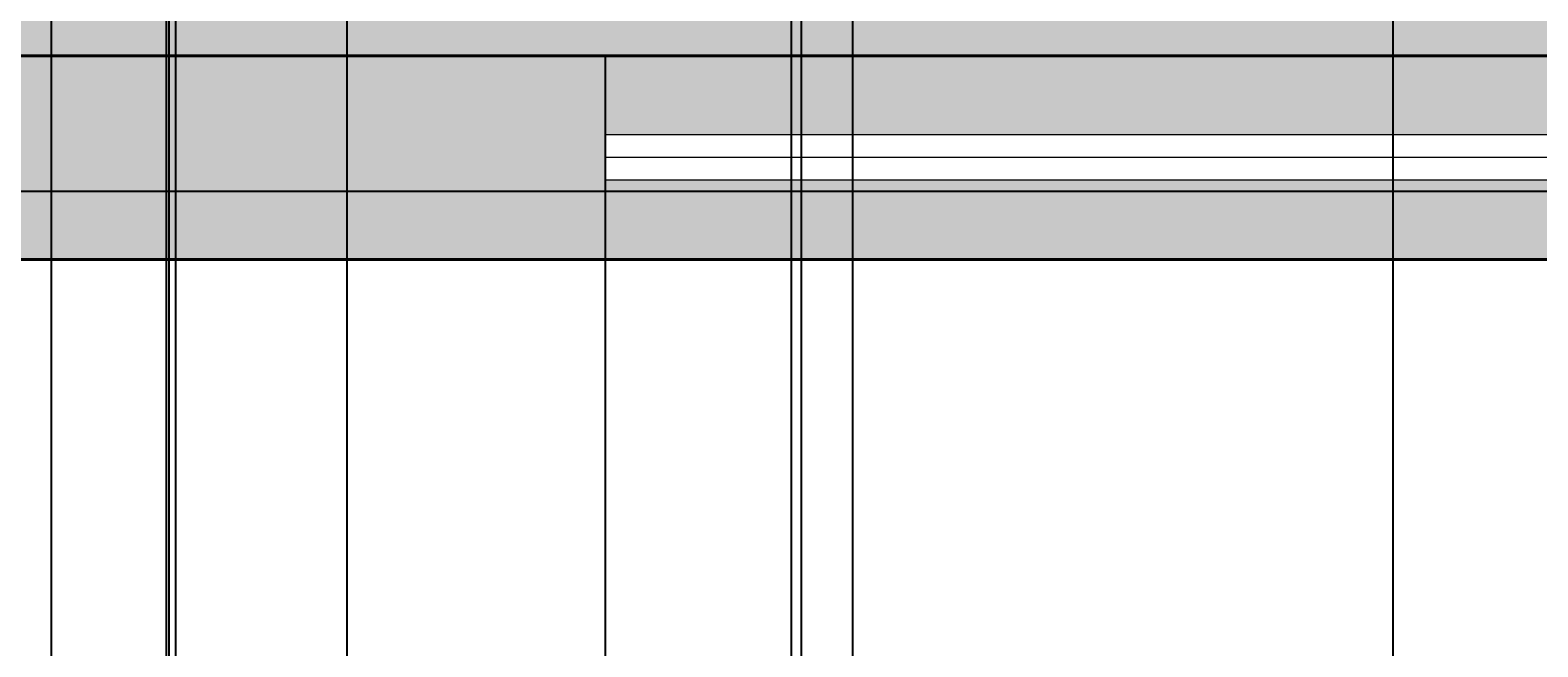
# Model space of a CAD drawing. Units: inches. Extents: x 818 to 1898, y 976 to 2364.
# Tile 74 of 96: x 1305 to 1372, y 2027 to 2054. Entities that reach past the tile are written whole.
import ezdxf

# ---------------------------------------------------------------- set-up
doc = ezdxf.new("R2010")
doc.units = ezdxf.units.IN
doc.header["$LTSCALE"] = 5
doc.header["$MEASUREMENT"] = 0
doc.linetypes.add('HIDDEN', pattern=[0.375, 0.25, -0.125])
for name, color, linetype, lineweight in [('A-ANNO-DIMS', 2, 'Continuous', 18), ('A-FLOR-OVHD', 8, 'HIDDEN', 13), ('A-GLAZ', 4, 'Continuous', 18), ('A-WALL', 7, 'Continuous', 40)]:
    doc.layers.add(name, color=color, linetype=linetype, lineweight=lineweight)
for name, color, linetype, lineweight, true_color in [('A-GLAZ-PATT', 141, 'Continuous', 9, 0xadddf7), ('A-WALL-PATT', 251, 'Continuous', 13, 0x636466), ('L-PLNT-PATT', 114, 'Continuous', 9, 0x139b48)]:
    doc.layers.add(name, color=color, linetype=linetype, lineweight=lineweight, true_color=true_color)
doc.styles.get("Standard").update_dxf_attribs({"font": 'arial.ttf'})
doc.dimstyles.get("Standard").update_dxf_attribs({"dimtxt": 0.18, "dimasz": 0.18, "dimexe": 0.18, "dimexo": 0.0625, "dimgap": 0.09, "dimtad": 0, "dimtih": 1, "dimtoh": 1, "dimdec": 4, "dimzin": 0, "dimdsep": 46, "dimtxsty": 'Standard', "dimcen": 0.09, "dimadec": 0, "dimazin": 0, "dimtfac": 1, "dimtdec": 4, "dimtofl": 0, "dimtmove": 0, "dimatfit": 3, "dimfxl": 1, "dimtolj": 1, "dimtzin": 0, "dimarcsym": 0})

# ---------------------------------------------------------------- blocks, each defined once
blk = doc.blocks.new('*D61')
at = {"layer": 'A-ANNO-DIMS', "color": 0, "lineweight": -2, "ltscale": 5, "transparency": 16777216}
for p, q in [((1071.725, 1203.027), (1071.725, 2363.873)), ((1071.905, 2363.693), (1250.936, 2363.693)), ((1430.545, 2363.693), (1251.514, 2363.693)), ((1430.725, 1203.027), (1430.725, 2363.873))]:
    blk.add_line(p, q, dxfattribs=at)
at = {"layer": 'A-ANNO-DIMS', "color": 0, "ltscale": 5, "transparency": 16777216}
for points in [[(1071.905, 2363.723), (1071.905, 2363.663), (1071.725, 2363.693)], [(1430.545, 2363.723), (1430.545, 2363.663), (1430.725, 2363.693)]]:
    blk.add_solid(points, dxfattribs=at)
at = {"layer": 'Defpoints', "color": 0, "ltscale": 5, "transparency": 16777216}
for p in [(1430.725, 2363.693), (1071.725, 1202.964), (1430.725, 1202.964)]:
    blk.add_point(p, dxfattribs=at)
at = {"layer": 'A-ANNO-DIMS', "color": 0, "ltscale": 5, "transparency": 16777216, "insert": (1251.225, 2363.693), "char_height": 0.18, "attachment_point": 5}
blk.add_mtext('\\A1;359', dxfattribs=at)
blk = doc.blocks.new('*D64')
at = {"layer": 'A-ANNO-DIMS', "color": 0, "lineweight": -2, "ltscale": 5, "transparency": 16777216}
for p, q in [((1197.725, 1501.141), (1197.725, 2363.873)), ((1197.905, 2363.693), (1313.935, 2363.693)), ((1430.545, 2363.693), (1314.516, 2363.693)), ((1430.725, 1501.141), (1430.725, 2363.873))]:
    blk.add_line(p, q, dxfattribs=at)
at = {"layer": 'A-ANNO-DIMS', "color": 0, "ltscale": 5, "transparency": 16777216}
for points in [[(1197.905, 2363.723), (1197.905, 2363.663), (1197.725, 2363.693)], [(1430.545, 2363.723), (1430.545, 2363.663), (1430.725, 2363.693)]]:
    blk.add_solid(points, dxfattribs=at)
at = {"layer": 'Defpoints', "color": 0, "ltscale": 5, "transparency": 16777216}
for p in [(1430.725, 2363.693), (1197.725, 1501.078), (1430.725, 1501.078)]:
    blk.add_point(p, dxfattribs=at)
at = {"layer": 'A-ANNO-DIMS', "color": 0, "ltscale": 5, "transparency": 16777216, "insert": (1314.225, 2363.693), "char_height": 0.18, "attachment_point": 5}
blk.add_mtext('\\A1;233', dxfattribs=at)
blk = doc.blocks.new('*D85')
at = {"layer": 'A-ANNO-DIMS', "color": 0, "lineweight": -2, "ltscale": 5, "transparency": 16777216}
for p, q in [((1258.788, 2053.078), (1897.916, 2053.078)), ((1897.736, 2052.898), (1897.736, 1876.76)), ((1897.736, 1700.258), (1897.736, 1876.396)), ((1258.788, 1700.078), (1897.916, 1700.078))]:
    blk.add_line(p, q, dxfattribs=at)
at = {"layer": 'A-ANNO-DIMS', "color": 0, "ltscale": 5, "transparency": 16777216}
for points in [[(1897.706, 2052.898), (1897.766, 2052.898), (1897.736, 2053.078)], [(1897.706, 1700.258), (1897.766, 1700.258), (1897.736, 1700.078)]]:
    blk.add_solid(points, dxfattribs=at)
at = {"layer": 'Defpoints', "color": 0, "ltscale": 5, "transparency": 16777216}
for p in [(1258.725, 2053.078), (1897.736, 2053.078), (1258.725, 1700.078)]:
    blk.add_point(p, dxfattribs=at)
at = {"layer": 'A-ANNO-DIMS', "color": 0, "ltscale": 5, "transparency": 16777216, "insert": (1897.736, 1876.578), "char_height": 0.18, "attachment_point": 5}
blk.add_mtext('\\A1;353', dxfattribs=at)
blk = doc.blocks.new('*D86')
at = {"layer": 'A-ANNO-DIMS', "color": 0, "lineweight": -2, "ltscale": 5, "transparency": 16777216}
for p, q in [((1258.725, 2053.141), (1258.725, 2363.873)), ((1258.905, 2363.693), (1486.433, 2363.693)), ((1714.545, 2363.693), (1487.018, 2363.693)), ((1714.725, 2053.141), (1714.725, 2363.873))]:
    blk.add_line(p, q, dxfattribs=at)
at = {"layer": 'A-ANNO-DIMS', "color": 0, "ltscale": 5, "transparency": 16777216}
for points in [[(1258.905, 2363.723), (1258.905, 2363.663), (1258.725, 2363.693)], [(1714.545, 2363.723), (1714.545, 2363.663), (1714.725, 2363.693)]]:
    blk.add_solid(points, dxfattribs=at)
at = {"layer": 'Defpoints', "color": 0, "ltscale": 5, "transparency": 16777216}
for p in [(1714.725, 2363.693), (1258.725, 2053.078), (1714.725, 2053.078)]:
    blk.add_point(p, dxfattribs=at)
at = {"layer": 'A-ANNO-DIMS', "color": 0, "ltscale": 5, "transparency": 16777216, "insert": (1486.725, 2363.693), "char_height": 0.18, "attachment_point": 5}
blk.add_mtext('\\A1;456', dxfattribs=at)
blk = doc.blocks.new('*D97')
at = {"layer": 'A-ANNO-DIMS', "color": 0, "lineweight": -2, "ltscale": 5, "transparency": 16777216}
for p, q in [((1284.17, 1071.118), (1284.17, 2363.873)), ((1284.35, 2363.693), (1310.962, 2363.693)), ((1338.361, 2363.693), (1311.749, 2363.693)), ((1338.541, 1071.118), (1338.541, 2363.873))]:
    blk.add_line(p, q, dxfattribs=at)
at = {"layer": 'A-ANNO-DIMS', "color": 0, "ltscale": 5, "transparency": 16777216}
for points in [[(1284.35, 2363.723), (1284.35, 2363.663), (1284.17, 2363.693)], [(1338.361, 2363.723), (1338.361, 2363.663), (1338.541, 2363.693)]]:
    blk.add_solid(points, dxfattribs=at)
at = {"layer": 'Defpoints', "color": 0, "ltscale": 5, "transparency": 16777216}
for p in [(1338.541, 2363.693), (1284.17, 1071.055), (1338.541, 1071.055)]:
    blk.add_point(p, dxfattribs=at)
at = {"layer": 'A-ANNO-DIMS', "color": 0, "ltscale": 5, "transparency": 16777216, "insert": (1311.355, 2363.693), "char_height": 0.18, "attachment_point": 5}
blk.add_mtext('\\A1;54.37', dxfattribs=at)
blk = doc.blocks.new('*D98')
at = {"layer": 'A-ANNO-DIMS', "color": 0, "lineweight": -2, "ltscale": 5, "transparency": 16777216}
for p, q in [((1338.541, 1071.118), (1338.541, 2363.873)), ((1338.721, 2363.693), (1364.815, 2363.693)), ((1391.696, 2363.693), (1365.602, 2363.693)), ((1391.876, 1071.118), (1391.876, 2363.873))]:
    blk.add_line(p, q, dxfattribs=at)
at = {"layer": 'A-ANNO-DIMS', "color": 0, "ltscale": 5, "transparency": 16777216}
for points in [[(1338.721, 2363.723), (1338.721, 2363.663), (1338.541, 2363.693)], [(1391.696, 2363.723), (1391.696, 2363.663), (1391.876, 2363.693)]]:
    blk.add_solid(points, dxfattribs=at)
at = {"layer": 'Defpoints', "color": 0, "ltscale": 5, "transparency": 16777216}
for p in [(1391.876, 2363.693), (1338.541, 1071.055), (1391.876, 1071.055)]:
    blk.add_point(p, dxfattribs=at)
at = {"layer": 'A-ANNO-DIMS', "color": 0, "ltscale": 5, "transparency": 16777216, "insert": (1365.208, 2363.693), "char_height": 0.18, "attachment_point": 5}
blk.add_mtext('\\A1;53.33', dxfattribs=at)
blk = doc.blocks.new('*D165')
at = {"layer": 'A-ANNO-DIMS', "color": 0, "lineweight": -2, "ltscale": 5, "transparency": 16777216}
for p, q in [((1283.818, 1510.141), (1283.818, 2363.873)), ((1283.998, 2363.693), (1324.088, 2363.693)), ((1364.966, 2363.693), (1324.876, 2363.693)), ((1365.146, 1510.141), (1365.146, 2363.873))]:
    blk.add_line(p, q, dxfattribs=at)
at = {"layer": 'A-ANNO-DIMS', "color": 0, "ltscale": 5, "transparency": 16777216}
for points in [[(1283.998, 2363.723), (1283.998, 2363.663), (1283.818, 2363.693)], [(1364.966, 2363.723), (1364.966, 2363.663), (1365.146, 2363.693)]]:
    blk.add_solid(points, dxfattribs=at)
at = {"layer": 'Defpoints', "color": 0, "ltscale": 5, "transparency": 16777216}
for p in [(1365.146, 2363.693), (1283.818, 1510.078), (1365.146, 1510.078)]:
    blk.add_point(p, dxfattribs=at)
at = {"layer": 'A-ANNO-DIMS', "color": 0, "ltscale": 5, "transparency": 16777216, "insert": (1324.482, 2363.693), "char_height": 0.18, "attachment_point": 5}
blk.add_mtext('\\A1;81.33', dxfattribs=at)
blk = doc.blocks.new('*D207')
at = {"layer": 'A-ANNO-DIMS', "color": 0, "lineweight": -2, "ltscale": 5, "transparency": 16777216}
for p, q in [((1590.663, 2044.078), (818.026, 2044.078)), ((818.206, 2043.898), (818.206, 2027.76)), ((818.206, 2011.258), (818.206, 2027.396)), ((1590.663, 2011.078), (818.026, 2011.078))]:
    blk.add_line(p, q, dxfattribs=at)
at = {"layer": 'A-ANNO-DIMS', "color": 0, "ltscale": 5, "transparency": 16777216}
for points in [[(818.176, 2043.898), (818.236, 2043.898), (818.206, 2044.078)], [(818.176, 2011.258), (818.236, 2011.258), (818.206, 2011.078)]]:
    blk.add_solid(points, dxfattribs=at)
at = {"layer": 'Defpoints', "color": 0, "ltscale": 5, "transparency": 16777216}
for p in [(818.206, 2044.078), (1590.725, 2044.078), (1590.725, 2011.078)]:
    blk.add_point(p, dxfattribs=at)
at = {"layer": 'A-ANNO-DIMS', "color": 0, "ltscale": 5, "transparency": 16777216, "insert": (818.206, 2027.578), "char_height": 0.18, "attachment_point": 5}
blk.add_mtext('\\A1;33', dxfattribs=at)
blk = doc.blocks.new('*D235')
at = {"layer": 'A-ANNO-DIMS', "color": 0, "lineweight": -2, "ltscale": 5, "transparency": 16777216}
for p, q in [((1310.908, 2026.27), (1310.908, 2363.873)), ((1311.088, 2363.693), (1324.485, 2363.693)), ((1338.812, 2363.693), (1325.414, 2363.693)), ((1338.992, 2026.27), (1338.992, 2363.873))]:
    blk.add_line(p, q, dxfattribs=at)
at = {"layer": 'A-ANNO-DIMS', "color": 0, "ltscale": 5, "transparency": 16777216}
for points in [[(1311.088, 2363.723), (1311.088, 2363.663), (1310.908, 2363.693)], [(1338.812, 2363.723), (1338.812, 2363.663), (1338.992, 2363.693)]]:
    blk.add_solid(points, dxfattribs=at)
at = {"layer": 'Defpoints', "color": 0, "ltscale": 5, "transparency": 16777216}
for p in [(1338.992, 2363.693), (1310.908, 2026.207), (1338.992, 2026.207)]:
    blk.add_point(p, dxfattribs=at)
at = {"layer": 'A-ANNO-DIMS', "color": 0, "ltscale": 5, "transparency": 16777216, "insert": (1324.95, 2363.693), "char_height": 0.18, "attachment_point": 5}
blk.add_mtext('\\A1;28.084', dxfattribs=at)
blk = doc.blocks.new('*D252')
at = {"layer": 'A-ANNO-DIMS', "color": 0, "lineweight": -2, "ltscale": 5, "transparency": 16777216}
for p, q in [((1330.305, 2053.016), (1330.305, 975.663)), ((1388.031, 2053.016), (1388.031, 975.663)), ((1330.485, 975.843), (1358.775, 975.843)), ((1387.851, 975.843), (1359.562, 975.843))]:
    blk.add_line(p, q, dxfattribs=at)
at = {"layer": 'A-ANNO-DIMS', "color": 0, "ltscale": 5, "transparency": 16777216}
for points in [[(1330.485, 975.873), (1330.485, 975.813), (1330.305, 975.843)], [(1387.851, 975.873), (1387.851, 975.813), (1388.031, 975.843)]]:
    blk.add_solid(points, dxfattribs=at)
at = {"layer": 'Defpoints', "color": 0, "ltscale": 5, "transparency": 16777216}
for p in [(1330.305, 2053.078), (1388.031, 2053.078), (1388.031, 975.843)]:
    blk.add_point(p, dxfattribs=at)
at = {"layer": 'A-ANNO-DIMS', "color": 0, "ltscale": 5, "transparency": 16777216, "insert": (1359.168, 975.843), "char_height": 0.18, "attachment_point": 5}
blk.add_mtext('\\A1;57.73', dxfattribs=at)
blk = doc.blocks.new('*D254')
at = {"layer": 'A-ANNO-DIMS', "color": 0, "lineweight": -2, "ltscale": 5, "transparency": 16777216}
for p, q in [((1267.725, 2044.016), (1267.725, 975.663)), ((1330.305, 2044.016), (1330.305, 975.663)), ((1267.905, 975.843), (1298.621, 975.843)), ((1330.125, 975.843), (1299.409, 975.843))]:
    blk.add_line(p, q, dxfattribs=at)
at = {"layer": 'A-ANNO-DIMS', "color": 0, "ltscale": 5, "transparency": 16777216}
for points in [[(1267.905, 975.873), (1267.905, 975.813), (1267.725, 975.843)], [(1330.125, 975.873), (1330.125, 975.813), (1330.305, 975.843)]]:
    blk.add_solid(points, dxfattribs=at)
at = {"layer": 'Defpoints', "color": 0, "ltscale": 5, "transparency": 16777216}
for p in [(1267.725, 2044.078), (1330.305, 2044.078), (1330.305, 975.843)]:
    blk.add_point(p, dxfattribs=at)
at = {"layer": 'A-ANNO-DIMS', "color": 0, "ltscale": 5, "transparency": 16777216, "insert": (1299.015, 975.843), "char_height": 0.18, "attachment_point": 5}
blk.add_mtext('\\A1;62.58', dxfattribs=at)
blk = doc.blocks.new('*D257')
at = {"layer": 'A-ANNO-DIMS', "color": 0, "lineweight": -2, "ltscale": 5, "transparency": 16777216}
for p, q in [((1399.573, 2077.188), (818.026, 2077.188)), ((818.206, 2077.008), (818.206, 2065.314)), ((818.206, 2053.258), (818.206, 2064.953)), ((1399.573, 2053.078), (818.026, 2053.078))]:
    blk.add_line(p, q, dxfattribs=at)
at = {"layer": 'A-ANNO-DIMS', "color": 0, "ltscale": 5, "transparency": 16777216}
for points in [[(818.176, 2077.008), (818.236, 2077.008), (818.206, 2077.188)], [(818.176, 2053.258), (818.236, 2053.258), (818.206, 2053.078)]]:
    blk.add_solid(points, dxfattribs=at)
at = {"layer": 'Defpoints', "color": 0, "ltscale": 5, "transparency": 16777216}
for p in [(818.206, 2077.188), (1399.636, 2077.188), (1399.636, 2053.078)]:
    blk.add_point(p, dxfattribs=at)
at = {"layer": 'A-ANNO-DIMS', "color": 0, "ltscale": 5, "transparency": 16777216, "insert": (818.206, 2065.133), "char_height": 0.18, "attachment_point": 5}
blk.add_mtext('\\A1;24.11', dxfattribs=at)
blk = doc.blocks.new('*D266')
at = {"layer": 'A-ANNO-DIMS', "color": 0, "lineweight": -2, "ltscale": 5, "transparency": 16777216}
for p, q in [((1780.439, 2053.078), (818.026, 2053.078)), ((818.206, 2052.898), (818.206, 2050.26)), ((818.206, 2047.258), (818.206, 2049.896)), ((1780.439, 2047.078), (818.026, 2047.078))]:
    blk.add_line(p, q, dxfattribs=at)
at = {"layer": 'A-ANNO-DIMS', "color": 0, "ltscale": 5, "transparency": 16777216}
for points in [[(818.176, 2052.898), (818.236, 2052.898), (818.206, 2053.078)], [(818.176, 2047.258), (818.236, 2047.258), (818.206, 2047.078)]]:
    blk.add_solid(points, dxfattribs=at)
at = {"layer": 'Defpoints', "color": 0, "ltscale": 5, "transparency": 16777216}
for p in [(1780.502, 2053.078), (818.206, 2047.078), (1780.502, 2047.078)]:
    blk.add_point(p, dxfattribs=at)
at = {"layer": 'A-ANNO-DIMS', "color": 0, "ltscale": 5, "transparency": 16777216, "insert": (818.206, 2050.078), "char_height": 0.18, "attachment_point": 5}
blk.add_mtext('\\A1;6', dxfattribs=at)
blk = doc.blocks.new('*D269')
at = {"layer": 'A-ANNO-DIMS', "color": 0, "lineweight": -2, "ltscale": 5, "transparency": 16777216}
for p, q in [((1246.938, 1534.141), (1246.938, 2363.873)), ((1247.118, 2363.693), (1293.706, 2363.693)), ((1341.079, 2363.693), (1294.491, 2363.693)), ((1341.259, 1534.141), (1341.259, 2363.873))]:
    blk.add_line(p, q, dxfattribs=at)
at = {"layer": 'A-ANNO-DIMS', "color": 0, "ltscale": 5, "transparency": 16777216}
for points in [[(1247.118, 2363.723), (1247.118, 2363.663), (1246.938, 2363.693)], [(1341.079, 2363.723), (1341.079, 2363.663), (1341.259, 2363.693)]]:
    blk.add_solid(points, dxfattribs=at)
at = {"layer": 'Defpoints', "color": 0, "ltscale": 5, "transparency": 16777216}
for p in [(1341.259, 2363.693), (1246.938, 1534.078), (1341.259, 1534.078)]:
    blk.add_point(p, dxfattribs=at)
at = {"layer": 'A-ANNO-DIMS', "color": 0, "ltscale": 5, "transparency": 16777216, "insert": (1294.099, 2363.693), "char_height": 0.18, "attachment_point": 5}
blk.add_mtext('\\A1;94.32', dxfattribs=at)
blk = doc.blocks.new('*D274')
at = {"layer": 'A-ANNO-DIMS', "color": 0, "lineweight": -2, "ltscale": 5, "transparency": 16777216}
for p, q in [((1311.025, 1897.929), (1311.025, 2363.873)), ((1311.205, 2363.693), (1344.007, 2363.693)), ((1377.599, 2363.693), (1344.797, 2363.693)), ((1377.779, 1897.929), (1377.779, 2363.873))]:
    blk.add_line(p, q, dxfattribs=at)
at = {"layer": 'A-ANNO-DIMS', "color": 0, "ltscale": 5, "transparency": 16777216}
for points in [[(1311.205, 2363.723), (1311.205, 2363.663), (1311.025, 2363.693)], [(1377.599, 2363.723), (1377.599, 2363.663), (1377.779, 2363.693)]]:
    blk.add_solid(points, dxfattribs=at)
at = {"layer": 'Defpoints', "color": 0, "ltscale": 5, "transparency": 16777216}
for p in [(1377.779, 2363.693), (1311.025, 1897.866), (1377.779, 1897.866)]:
    blk.add_point(p, dxfattribs=at)
at = {"layer": 'A-ANNO-DIMS', "color": 0, "ltscale": 5, "transparency": 16777216, "insert": (1344.402, 2363.693), "char_height": 0.18, "attachment_point": 5}
blk.add_mtext('\\A1;66.75', dxfattribs=at)
blk = doc.blocks.new('*D281')
at = {"layer": 'A-ANNO-DIMS', "color": 0, "lineweight": -2, "ltscale": 5, "transparency": 16777216}
for p, q in [((1250.303, 1913.703), (1250.303, 2363.873)), ((1250.483, 2363.693), (1420.121, 2363.693)), ((1590.545, 2363.693), (1420.907, 2363.693)), ((1590.725, 2011.141), (1590.725, 2363.873))]:
    blk.add_line(p, q, dxfattribs=at)
at = {"layer": 'A-ANNO-DIMS', "color": 0, "ltscale": 5, "transparency": 16777216}
for points in [[(1250.483, 2363.723), (1250.483, 2363.663), (1250.303, 2363.693)], [(1590.545, 2363.723), (1590.545, 2363.663), (1590.725, 2363.693)]]:
    blk.add_solid(points, dxfattribs=at)
at = {"layer": 'Defpoints', "color": 0, "ltscale": 5, "transparency": 16777216}
for p in [(1590.725, 2363.693), (1590.725, 2011.078), (1250.303, 1913.64)]:
    blk.add_point(p, dxfattribs=at)
at = {"layer": 'A-ANNO-DIMS', "color": 0, "ltscale": 5, "transparency": 16777216, "insert": (1420.514, 2363.693), "char_height": 0.18, "attachment_point": 5}
blk.add_mtext('\\A1;340.4', dxfattribs=at)
blk = doc.blocks.new('*D286')
at = {"layer": 'A-ANNO-DIMS', "color": 0, "lineweight": -2, "ltscale": 5, "transparency": 16777216}
for p, q in [((1305.828, 1851.971), (1305.828, 2363.873)), ((1306.008, 2363.693), (1308.184, 2363.693)), ((1311.147, 2363.693), (1308.971, 2363.693)), ((1311.327, 1853.812), (1311.327, 2363.873))]:
    blk.add_line(p, q, dxfattribs=at)
at = {"layer": 'A-ANNO-DIMS', "color": 0, "ltscale": 5, "transparency": 16777216}
for points in [[(1306.008, 2363.723), (1306.008, 2363.663), (1305.828, 2363.693)], [(1311.147, 2363.723), (1311.147, 2363.663), (1311.327, 2363.693)]]:
    blk.add_solid(points, dxfattribs=at)
at = {"layer": 'Defpoints', "color": 0, "ltscale": 5, "transparency": 16777216}
for p in [(1305.828, 2363.693), (1311.327, 1853.75), (1305.828, 1851.908)]:
    blk.add_point(p, dxfattribs=at)
at = {"layer": 'A-ANNO-DIMS', "color": 0, "ltscale": 5, "transparency": 16777216, "insert": (1308.577, 2363.693), "char_height": 0.18, "attachment_point": 5}
blk.add_mtext('\\A1;5.499', dxfattribs=at)
blk = doc.blocks.new('*D290')
at = {"layer": 'A-ANNO-DIMS', "color": 0, "lineweight": -2, "ltscale": 5, "transparency": 16777216}
for p, q in [((1302.983, 1599.435), (1302.983, 2363.873)), ((1303.163, 2363.693), (1310.57, 2363.693)), ((1318.713, 2363.693), (1311.306, 2363.693)), ((1318.893, 1607.833), (1318.893, 2363.873))]:
    blk.add_line(p, q, dxfattribs=at)
at = {"layer": 'A-ANNO-DIMS', "color": 0, "ltscale": 5, "transparency": 16777216}
for points in [[(1303.163, 2363.723), (1303.163, 2363.663), (1302.983, 2363.693)], [(1318.713, 2363.723), (1318.713, 2363.663), (1318.893, 2363.693)]]:
    blk.add_solid(points, dxfattribs=at)
at = {"layer": 'Defpoints', "color": 0, "ltscale": 5, "transparency": 16777216}
for p in [(1318.893, 2363.693), (1318.893, 1607.771), (1302.983, 1599.372)]:
    blk.add_point(p, dxfattribs=at)
at = {"layer": 'A-ANNO-DIMS', "color": 0, "ltscale": 5, "transparency": 16777216, "insert": (1310.938, 2363.693), "char_height": 0.18, "attachment_point": 5}
blk.add_mtext('\\A1;15.91', dxfattribs=at)

msp = doc.modelspace()

# ---------------------------------------------------------------- hatches: boundary and pattern name
at = {"layer": 'A-GLAZ-PATT', "ltscale": 5}
h = msp.add_hatch(color=256, dxfattribs=at)
h.dxf.hatch_style = 1
h.paths.add_polyline_path([(1283.8183, 1504.5782), (1206.7252, 1504.5782), (1206.7252, 1501.0782), (1283.8183, 1501.0782)])
h.paths.add_polyline_path([(1283.8183, 1510.0782), (1206.7252, 1510.0782), (1206.7252, 1506.5782), (1283.8183, 1506.5782)])
h.paths.add_polyline_path([(1490.9163, 1355.0782), (1439.7252, 1355.0782), (1439.7252, 1409.0522), (1436.2252, 1409.0522), (1436.2252, 1351.5782), (1490.9163, 1351.5782)])
h.paths.add_polyline_path([(1434.2252, 1409.0522), (1430.7251, 1409.0522), (1430.7251, 1346.0782), (1435.0799, 1346.0782), (1435.0731, 1346.1152), (1435.1501, 1346.0782), (1490.9163, 1346.0782), (1490.9163, 1349.5782), (1434.2252, 1349.5782)])
h.paths.add_polyline_path([(1714.7251, 1545.0782), (1711.2252, 1545.0782), (1711.2252, 1521.0782), (1714.7251, 1521.0782)])
h.paths.add_polyline_path([(1709.2252, 1545.0782), (1705.7252, 1545.0782), (1705.7252, 1521.0782), (1709.2252, 1521.0782)])
h.paths.add_polyline_path([(1714.7251, 1687.0782), (1711.2252, 1687.0782), (1711.2252, 1649.9029), (1714.7251, 1649.9029)])
h.paths.add_polyline_path([(1709.2252, 1687.0782), (1705.7252, 1687.0782), (1705.7252, 1649.9029), (1709.2252, 1649.9029)])
h.paths.add_polyline_path([(1709.2252, 1745.5584), (1705.7252, 1745.5584), (1705.7252, 1717.3178), (1709.2252, 1717.3178)])
h.paths.add_polyline_path([(1714.7251, 1745.5584), (1711.2252, 1745.5584), (1711.2252, 1717.3178), (1714.7251, 1717.3178)])
h.paths.add_polyline_path([(1714.7251, 2014.5114), (1711.2252, 2014.5114), (1711.2252, 1962.0338), (1714.7251, 1962.0338)])
h.paths.add_polyline_path([(1709.2252, 2014.5114), (1705.7252, 2014.5114), (1705.7252, 1962.0338), (1709.2252, 1962.0338)])
h.paths.add_polyline_path([(1538.5155, 2047.5782), (1485.1216, 2047.5782), (1485.1216, 2044.0782), (1538.5155, 2044.0782)])
h.paths.add_polyline_path([(1538.5155, 2053.0782), (1485.1216, 2053.0782), (1485.1216, 2049.5782), (1538.5155, 2049.5782)])
h.paths.add_polyline_path([(1388.0315, 2047.5782), (1330.305, 2047.5782), (1330.305, 2044.0782), (1388.0315, 2044.0782)])
h.paths.add_polyline_path([(1388.0315, 2053.0782), (1330.305, 2053.0782), (1330.305, 2049.5782), (1388.0315, 2049.5782)])
h.paths.add_polyline_path([(1262.2252, 2019.2871), (1258.7251, 2019.2871), (1258.7251, 1928.9218), (1262.2252, 1928.9218)])
h.paths.add_polyline_path([(1267.7251, 2019.2871), (1264.2252, 2019.2871), (1264.2252, 1928.9218), (1267.7251, 1928.9218)])
h.paths.add_polyline_path([(1262.2252, 1862.9652), (1258.7251, 1862.9652), (1258.7251, 1814.9652), (1262.2252, 1814.9652)])
h.paths.add_polyline_path([(1267.7251, 1862.9652), (1264.2252, 1862.9652), (1264.2252, 1814.9652), (1267.7251, 1814.9652)])
h.paths.add_polyline_path([(1262.2252, 1755.3321), (1258.7251, 1755.3321), (1258.7251, 1707.3321), (1262.2252, 1707.3321)])
h.paths.add_polyline_path([(1267.7251, 1755.3321), (1264.2252, 1755.3321), (1264.2252, 1707.3321), (1267.7251, 1707.3321)])
h.paths.add_polyline_path([(1251.9333, 1692.5782), (1206.7252, 1692.5782), (1206.7252, 1687.0782), (1251.9333, 1687.0782)])
h.paths.add_polyline_path([(1251.9333, 1700.0782), (1206.7252, 1700.0782), (1206.7252, 1694.5782), (1251.9333, 1694.5782)])
at = {"layer": 'A-WALL-PATT', "ltscale": 5}
h = msp.add_hatch(color=256, dxfattribs=at)
h.dxf.hatch_style = 1
h.paths.add_polyline_path([(1267.7251, 1928.9218), (1258.7251, 1928.9218), (1258.7251, 1913.6401), (1250.3029, 1913.6401), (1250.3029, 1878.3919), (1258.7251, 1878.3919), (1258.7251, 1862.9652), (1267.7251, 1862.9652)])
h.paths.add_polyline_path([(1267.7251, 1814.9652), (1258.7251, 1814.9652), (1258.7251, 1755.3321), (1267.7251, 1755.3321)])
h.paths.add_polyline_path([(1463.7252, 1696.0782), (1267.7251, 1696.0782), (1267.7251, 1707.3321), (1258.7251, 1707.3321), (1258.7251, 1700.0782), (1251.9333, 1700.0782), (1251.9333, 1687.0782), (1463.7252, 1687.0782)])
h.paths.add_polyline_path([(1714.7251, 1717.3178), (1705.7252, 1717.3178), (1705.7252, 1696.0782), (1599.7252, 1696.0782), (1599.7252, 1790.0782), (1705.7252, 1790.0782), (1705.7252, 1785.6125), (1714.7251, 1785.6125), (1714.7251, 1827.2125), (1705.7252, 1827.2125), (1705.7252, 1802.0782), (1599.7252, 1802.0782), (1599.7252, 1867.0782), (1705.7252, 1867.0782), (1705.7252, 1857.2125), (1714.7251, 1857.2125), (1714.7251, 1930.0316), (1741.8409, 1930.0316), (1741.8409, 1935.0316), (1714.7251, 1935.0316), (1714.7251, 1957.0338), (1741.8409, 1957.0338), (1741.8409, 1962.0338), (1714.7251, 1962.0338), (1705.7252, 1962.0338), (1705.7252, 1948.0782), (1599.7252, 1948.0782), (1599.7252, 1981.0782), (1590.7251, 1981.0782), (1590.7251, 1941.0782), (1620.7252, 1941.0782), (1705.7252, 1941.0782), (1705.7252, 1876.0782), (1599.7252, 1876.0782), (1599.7252, 1911.0782), (1590.7251, 1911.0782), (1590.7251, 1876.0782), (1429.2252, 1876.0782), (1429.2252, 1867.0782), (1511.7252, 1867.0782), (1528.593, 1867.0782), (1595.7252, 1867.0782), (1595.7252, 1773.0782), (1520.7252, 1773.0782), (1520.7252, 1837.5823), (1532.593, 1837.5823), (1532.593, 1867.0782), (1528.593, 1867.0782), (1528.593, 1841.5823), (1511.7252, 1841.5823), (1511.7252, 1744.9714), (1520.7252, 1744.9714), (1520.7252, 1761.0782), (1595.7252, 1761.0782), (1595.7252, 1696.0782), (1520.7252, 1696.0782), (1520.7252, 1716.0454), (1511.7252, 1716.0454), (1511.7252, 1696.0782), (1511.7252, 1687.0782), (1714.7251, 1687.0782)])
h.paths.add_polyline_path([(1714.7251, 2053.0782), (1714.7251, 2081.1881), (1709.7252, 2081.1881), (1709.7252, 2053.0782), (1681.6446, 2053.0782), (1681.6446, 2081.1881), (1676.6446, 2081.1881), (1676.6446, 2053.0782), (1538.5155, 2053.0782), (1538.5155, 2044.0782), (1590.7251, 2044.0782), (1590.7251, 2011.0782), (1599.7252, 2011.0782), (1599.7252, 2044.0782), (1705.7252, 2044.0782), (1705.7252, 2014.5114), (1714.7251, 2014.5114)])
h.paths.add_polyline_path([(1485.1216, 2053.0782), (1422.02, 2053.0782), (1422.02, 2081.1881), (1413.02, 2081.1881), (1413.02, 2053.0782), (1399.6356, 2053.0782), (1399.6356, 2081.1881), (1390.6356, 2081.1881), (1390.6356, 2053.0782), (1388.0315, 2053.0782), (1388.0315, 2044.0782), (1416.2743, 2044.0782), (1485.1216, 2044.0782)])
h.paths.add_polyline_path([(1330.305, 2053.0782), (1258.7251, 2053.0782), (1258.7251, 2019.2871), (1267.7251, 2019.2871), (1267.7251, 2044.0782), (1330.305, 2044.0782)])
h.paths.add_polyline_path([(1258.7251, 2053.0782), (1214.6577, 2053.0782), (1214.6577, 2044.0782), (1258.7251, 2044.0782)])
h.paths.add_polyline_path([(1214.6577, 2053.0782), (1180.349, 2053.0782), (1180.349, 2044.0782), (1214.6577, 2044.0782)])
h.paths.add_polyline_path([(1714.7251, 1639.5782), (1741.8409, 1639.5782), (1741.8409, 1643.5782), (1714.7251, 1643.5782), (1714.7251, 1649.9029), (1705.7252, 1649.9029), (1705.7252, 1600.0782), (1477.7252, 1600.0782), (1477.7252, 1591.0782), (1520.7252, 1591.0782), (1616.7252, 1591.0782), (1616.7252, 1416.6857), (1622.7252, 1416.6857), (1622.7252, 1463.0782), (1624.7252, 1463.0782), (1624.7252, 1467.0782), (1622.7252, 1467.0782), (1622.7252, 1591.0782), (1705.7252, 1591.0782), (1705.7252, 1545.0782), (1714.7251, 1545.0782), (1741.8409, 1545.0782), (1741.8409, 1549.0782), (1714.7251, 1549.0782), (1714.7251, 1593.9175), (1737.8409, 1593.9175), (1737.8409, 1597.9175), (1714.7251, 1597.9175)])
h.paths.add_polyline_path([(1674.9024, 2060.7419), (1714.7045, 2060.7419), (1714.7045, 2073.1061), (1674.9024, 2073.1061)], flags=25)
h.paths.add_polyline_path([(1394.5468, 2061.6618), (1422.2344, 2061.6618), (1422.2344, 2074.0261), (1394.5468, 2074.0261)], flags=24)
at = {"layer": 'L-PLNT-PATT', "ltscale": 5}
h = msp.add_hatch(color=256, dxfattribs=at)
h.dxf.hatch_style = 1
h.paths.add_polyline_path([(1789.7173, 2205.9709), (1083.7252, 2205.9709), (1083.7252, 2083.2623), (1218.1114, 2083.2623), (1218.1114, 2053.0782), (1390.6356, 2053.0782), (1390.6356, 2081.1881), (1399.6356, 2081.1881), (1413.02, 2081.1881), (1422.02, 2081.1881), (1422.02, 2053.0782), (1676.6446, 2053.0782), (1676.6446, 2081.1881), (1714.7251, 2081.1881), (1714.7251, 2081.6235), (1789.7173, 2081.6235)])
h.paths.add_polyline_path([(1388.6037, 2145.2461), (1388.6037, 2122.3767), (1373.4756, 2122.3767), (1373.4756, 2145.2461)], flags=16)
h.paths.add_polyline_path([(1408.6922, 2145.2461), (1423.8203, 2145.2461), (1423.8203, 2122.3767), (1408.6922, 2122.3767)], flags=16)
h.paths.add_polyline_path([(1353.3871, 2155.7839), (1353.3871, 2122.3767), (1338.259, 2122.3767), (1338.259, 2155.7839)], flags=16)
h.paths.add_polyline_path([(1443.9089, 2158.4222), (1459.037, 2158.4222), (1459.037, 2122.3767), (1443.9089, 2122.3767)], flags=16)
h.paths.add_polyline_path([(1318.1705, 2145.2461), (1318.1705, 2122.3767), (1303.0424, 2122.3767), (1303.0424, 2145.2461)], flags=16)
h.paths.add_polyline_path([(1479.1255, 2145.2461), (1494.2536, 2145.2461), (1494.2536, 2122.3767), (1479.1255, 2122.3767)], flags=16)
h.paths.add_polyline_path([(1282.9539, 2145.2461), (1282.9539, 2122.3767), (1267.8258, 2122.3767), (1267.8258, 2145.2461)], flags=16)
h.paths.add_polyline_path([(1514.3421, 2145.2461), (1529.4702, 2145.2461), (1529.4702, 2122.3767), (1514.3421, 2122.3767)], flags=16)
h.paths.add_polyline_path([(1247.7373, 2159.4296), (1247.7373, 2122.3767), (1232.6091, 2122.3767), (1232.6091, 2159.4296)], flags=16)
h.paths.add_polyline_path([(1549.5587, 2156.9246), (1564.6868, 2156.9246), (1564.6868, 2122.3767), (1549.5587, 2122.3767)], flags=16)
h.paths.add_polyline_path([(1212.5206, 2145.2461), (1212.5206, 2122.3767), (1197.3925, 2122.3767), (1197.3925, 2145.2461)], flags=16)
h.paths.add_polyline_path([(1584.7753, 2145.2461), (1599.9034, 2145.2461), (1599.9034, 2122.3767), (1584.7753, 2122.3767)], flags=16)
h.paths.add_polyline_path([(1185.1073, 2104.7786), (1190.6407, 2104.7786), (1185.1073, 2098.2505), (1179.5738, 2104.7786)], flags=16)
h.paths.add_polyline_path([(1619.9919, 2145.2461), (1635.1201, 2145.2461), (1635.1201, 2122.3767), (1619.9919, 2122.3767)], flags=16)
h.paths.add_polyline_path([(1655.2086, 2156.1761), (1670.3367, 2156.1761), (1670.3367, 2122.3767), (1655.2086, 2122.3767)], flags=16)
h.paths.add_polyline_path([(1686.5992, 2145.2461), (1701.7273, 2145.2461), (1701.7273, 2122.3767), (1686.5992, 2122.3767)], flags=16)
h.paths.add_polyline_path([(1715.7616, 2145.2461), (1730.8897, 2145.2461), (1730.8897, 2122.3767), (1715.7616, 2122.3767)], flags=16)
h.paths.add_polyline_path([(1753.1652, 2145.2461), (1776.3312, 2145.2461), (1776.3312, 2115.6891), (1753.1652, 2115.6891)], flags=16)
h.paths.add_polyline_path([(1191.4331, 2146.5159), (1176.7891, 2146.5159), (1176.7891, 2134.1516), (1191.4331, 2134.1516)], flags=24)

# ---------------------------------------------------------------- linework, layer by layer
at = {"layer": 'A-FLOR-OVHD', "ltscale": 5}
msp.add_lwpolyline([(1267.7251, 2044.0782), (1416.2743, 2044.0782), (1416.2743, 1918.9894), (1267.7251, 1918.9894)], close=True, dxfattribs=at)
at = {"layer": 'A-GLAZ'}
for p, q in [((1330.305, 2053.0782), (1330.305, 2044.0782)), ((1388.0315, 2049.5782), (1330.305, 2049.5782)), ((1388.0315, 2048.5782), (1330.305, 2048.5782)), ((1388.0315, 2047.5782), (1330.305, 2047.5782))]:
    msp.add_line(p, q, dxfattribs=at)
at = {"layer": 'A-WALL'}
for p, q in [((1083.7252, 2053.0782), (1390.6356, 2053.0782)), ((1267.7251, 2044.0782), (1590.7251, 2044.0782))]:
    msp.add_line(p, q, dxfattribs=at)

# ---------------------------------------------------------------- dimensions: what is measured, and where the dimension line sits
at = {"layer": 'A-ANNO-DIMS', "ltscale": 5}
for base, p1, p2, override, picture, middle in [((1430.7251, 2363.6929), (1071.7251, 1202.9642), (1430.7251, 1202.9642), {"dimdec": 0, "dimlfac": 1, "dimrnd": 0, "dimzin": 0, "dimdsep": 46, "dimlunit": 2}, '*D61', (1251.2251, 2363.6929)), ((1430.7251, 2363.6929), (1197.7251, 1501.0782), (1430.7251, 1501.0782), {"dimdec": 0, "dimlfac": 1, "dimrnd": 0, "dimzin": 0, "dimdsep": 46, "dimlunit": 2}, '*D64', (1314.2251, 2363.6929)), ((1341.2593, 2363.6929), (1246.9377, 1534.0782), (1341.2593, 1534.0782), {"dimdec": 2, "dimlfac": 1, "dimrnd": 0, "dimzin": 0, "dimdsep": 46, "dimlunit": 2}, '*D269', (1294.0985, 2363.6929)), ((1590.7251, 2363.6929), (1250.3029, 1913.6401), (1590.7251, 2011.0782), {"dimdec": 1, "dimlfac": 1, "dimrnd": 0, "dimzin": 0, "dimdsep": 46, "dimlunit": 2}, '*D281', (1420.514, 2363.6929)), ((1714.7251, 2363.6929), (1258.7251, 2053.0782), (1714.7251, 2053.0782), {"dimdec": 0, "dimlfac": 1, "dimrnd": 0, "dimzin": 0, "dimdsep": 46, "dimlunit": 2}, '*D86', (1486.7251, 2363.6929)), ((1365.1463, 2363.6929), (1283.8183, 1510.0782), (1365.1463, 1510.0782), {"dimdec": 2, "dimlfac": 1, "dimrnd": 0, "dimzin": 0, "dimdsep": 46, "dimlunit": 2}, '*D165', (1324.4823, 2363.6929)), ((1338.5412, 2363.6929), (1284.1697, 1071.0552), (1338.5412, 1071.0552), {"dimdec": 2, "dimlfac": 1, "dimrnd": 0, "dimzin": 0, "dimdsep": 46, "dimlunit": 2}, '*D97', (1311.3554, 2363.6929)), ((1318.8931, 2363.6929), (1302.9835, 1599.3725), (1318.8931, 1607.7707), {"dimdec": 2, "dimlfac": 1, "dimrnd": 0, "dimzin": 0, "dimdsep": 46, "dimlunit": 2}, '*D290', (1310.9383, 2363.6929)), ((1305.8278, 2363.6929), (1311.3271, 1853.7496), (1305.8278, 1851.9081), {"dimdec": 3, "dimlfac": 1, "dimrnd": 0, "dimzin": 0, "dimdsep": 46, "dimlunit": 2}, '*D286', (1308.5774, 2363.6929)), ((1338.9915, 2363.6929), (1310.9077, 2026.2074), (1338.9915, 2026.2074), {"dimdec": 3, "dimlfac": 1, "dimrnd": 0, "dimzin": 0, "dimdsep": 46, "dimlunit": 2}, '*D235', (1324.9496, 2363.6929)), ((1377.7791, 2363.6929), (1311.025, 1897.8663), (1377.7791, 1897.8663), {"dimdec": 2, "dimlfac": 1, "dimrnd": 0, "dimzin": 0, "dimdsep": 46, "dimlunit": 2}, '*D274', (1344.4021, 2363.6929)), ((1391.8757, 2363.6929), (1338.5412, 1071.0552), (1391.8757, 1071.0552), {"dimdec": 2, "dimlfac": 1, "dimrnd": 0, "dimzin": 0, "dimdsep": 46, "dimlunit": 2}, '*D98', (1365.2084, 2363.6929)), ((1388.0315, 975.8433), (1330.305, 2053.0782), (1388.0315, 2053.0782), {"dimdec": 2, "dimlfac": 1, "dimrnd": 0, "dimzin": 0, "dimdsep": 46, "dimlunit": 2}, '*D252', (1359.1682, 975.8433)), ((1330.305, 975.8433), (1267.7251, 2044.0782), (1330.305, 2044.0782), {"dimdec": 2, "dimlfac": 1, "dimrnd": 0, "dimzin": 0, "dimdsep": 46, "dimlunit": 2}, '*D254', (1299.0151, 975.8433))]:
    dim = msp.add_linear_dim(base=base, p1=p1, p2=p2, dimstyle='Standard', override=override, dxfattribs=at)
    dim.commit()
    dim.dimension.update_dxf_attribs({"geometry": picture, "text_midpoint": middle})
for base, p1, p2, override, picture, middle in [((818.2059, 2077.1881), (1399.6356, 2053.0782), (1399.6356, 2077.1881), {"dimdec": 2, "dimlfac": 1, "dimrnd": 0, "dimzin": 0, "dimdsep": 46, "dimlunit": 2}, '*D257', (818.2059, 2065.1332)), ((818.2059, 2047.0782), (1780.5019, 2053.0782), (1780.5019, 2047.0782), {"dimdec": 0, "dimlfac": 1, "dimrnd": 0, "dimzin": 0, "dimdsep": 46, "dimlunit": 2}, '*D266', (818.2059, 2050.0782)), ((1897.736, 2053.0782), (1258.7251, 1700.0782), (1258.7251, 2053.0782), {"dimdec": 0, "dimlfac": 1, "dimrnd": 0, "dimzin": 0, "dimdsep": 46, "dimlunit": 2}, '*D85', (1897.736, 1876.5782)), ((818.2059, 2044.0782), (1590.7251, 2011.0782), (1590.7251, 2044.0782), {"dimdec": 0, "dimlfac": 1, "dimrnd": 0, "dimzin": 0, "dimdsep": 46, "dimlunit": 2}, '*D207', (818.2059, 2027.5782))]:
    dim = msp.add_linear_dim(base=base, p1=p1, p2=p2, angle=90, dimstyle='Standard', override=override, dxfattribs=at)
    dim.commit()
    dim.dimension.update_dxf_attribs({"geometry": picture, "text_midpoint": middle})

doc.saveas('drawing.dxf')
